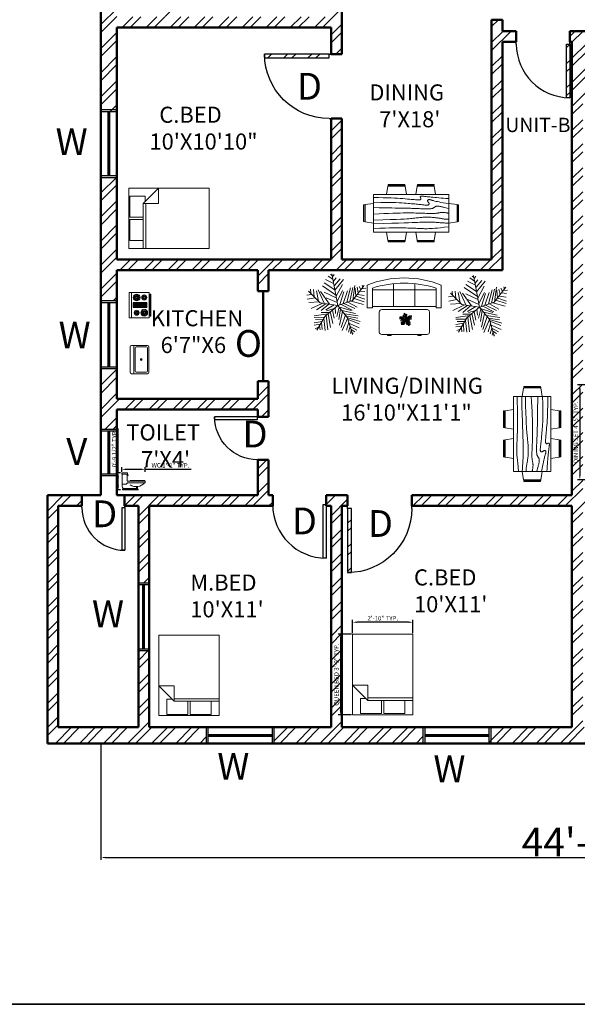
# Model space of a CAD drawing. Units: inches. Extents: x -31842 to -29388, y 18869 to 19743.
# Tile 10 of 12: x -30172 to -29859, y 18869 to 19420. Entities that reach past the tile are written whole.
import ezdxf

# ---------------------------------------------------------------- set-up
doc = ezdxf.new("R2010")
doc.units = ezdxf.units.IN
for name, color, linetype, lineweight in [('A-ANNO-DIMS', 2, 'Continuous', 18), ('A-ANNO-SYMB', 2, 'Continuous', 18), ('A-ANNO-TTLB', 7, 'Continuous', 35), ('A-AREA-IDEN', 3, 'Continuous', 18), ('A-DOOR', 3, 'Continuous', 25), ('A-FLOR-FIXT', 8, 'Continuous', 18), ('A-FURN', 8, 'Continuous', 18), ('A-GLAZ', 4, 'Continuous', 25), ('A-WALL', 7, 'Continuous', 50), ('A-WALL-PATT', 8, 'Continuous', 13), ('L-PLNT', 3, 'Continuous', 13)]:
    doc.layers.add(name, color=color, linetype=linetype, lineweight=lineweight)
doc.styles.get("Standard").update_dxf_attribs({"font": 'arial.ttf'})
doc.dimstyles.new('ISO-25', dxfattribs={"dimtxt": 2.5, "dimasz": 2.5, "dimexe": 1.25, "dimexo": 0.625, "dimtad": 1, "dimdec": 0, "dimlunit": 3, "dimtxsty": 'Standard', "dimcen": 2.5, "dimadec": 0, "dimazin": 0, "dimtfac": 1, "dimtdec": 0, "dimtmove": 0, "dimatfit": 3, "dimfxl": 1, "dimarcsym": 0})

# ---------------------------------------------------------------- blocks, each defined once
blk = doc.blocks.new('*U8')
for p, q in [((0, 0), (0, -100)), ((750, 0), (750, -100))]:
    blk.add_line(p, q)
blk.add_lwpolyline([(0, 0), (0, 750), (43.75, 750), (43.75, 0)], close=True)
blk.add_arc((0, 0), 750, 0, 90)
blk = doc.blocks.new('Bed - Queen')
for p, q in [((0, -80.00003), (0, 0)), ((0, 0), (59.99999, 0)), ((59.99999, 0), (59.99999, -80.00003)), ((7.99999, -1.2), (28.79998, -1.2)), ((7.99999, -14.4), (7.99999, -1.2)), ((28.79998, -1.2), (28.79998, -14.4)), ((31.19999, -1.2), (51.99999, -1.2)), ((31.19999, -14.4), (31.19999, -1.2)), ((51.99999, -1.2), (51.99999, -16.4)), ((0, -14.4), (44.8, -14.4)), ((44.8, -16.8), (0, -16.8)), ((59.99999, -29.6), (44.8, -14.4)), ((44.8, -14.4), (44.8, -29.6)), ((51.99999, -16.4), (46.79936, -16.4)), ((44.8, -29.6), (59.99999, -29.6)), ((59.99999, -80.00003), (0, -80.00003))]:
    blk.add_line(p, q)
blk = doc.blocks.new('Range-Oven - 30 in top')
for p, q in [((0, -3), (30, -3)), ((12, -6), (18, -6)), ((13, -20), (13, -6)), ((14, -6), (14, -20)), ((15, -20), (15, -6)), ((16, -6), (16, -20)), ((17, -20), (17, -6)), ((18, -20), (12, -20)), ((6, -24), (6, -25)), ((8, -25), (8, -24)), ((22, -25), (22, -24)), ((24, -24), (24, -25))]:
    blk.add_line(p, q)
for points in [[(0, -24), (0, 0), (30, 0), (30, -24)], [(12, -21), (12, -5), (18, -5), (18, -21)], [(2, -26), (2, -25), (28, -25), (28, -26)]]:
    blk.add_lwpolyline(points, close=True)
for centre, radius in [((6, -9), 4), ((6, -9), 3), ((6, -9), 2), ((6, -9), 1), ((24, -9), 3), ((24, -9), 2), ((24, -9), 1), ((6, -18), 3), ((6, -18), 2), ((6, -18), 1), ((24, -18), 4), ((24, -18), 3), ((24, -18), 2), ((24, -18), 1)]:
    blk.add_circle(centre, radius)
blk = doc.blocks.new('Sink-single - 30 in top')
blk.add_line((-15, -3.999996), (15, -3.999996))
for points in [[(-13.5, 0), (13.5, 0)], [(-15, -18.499996), (-15, -1.5)], [(-13.5, -17.499996), (-13.5, -6.499996)], [(-12.5, -5.499996), (12.5, -5.499996)], [(13.5, -6.499996), (13.5, -17.499996)], [(15, -1.5), (15, -18.499996)], [(13.5, -19.999996), (-13.5, -19.999996)], [(12.5, -18.499996), (-12.5, -18.499996)]]:
    blk.add_lwpolyline(points)
for radius in [1, 0.5]:
    blk.add_circle((0, -11.999996), radius)
for centre, radius, start, end in [((-13.5, -1.5), 1.5, 90, 180), ((-12.5, -6.499996), 1, 90, 180), ((12.5, -6.499996), 1, 0, 90), ((13.5, -1.5), 1.5, 0, 90), ((-13.5, -18.499996), 1.5, 180, 270), ((-12.5, -17.499996), 1, 180, 270), ((12.5, -17.499996), 1, 270, 0), ((13.5, -18.499996), 1.5, 270, 0)]:
    blk.add_arc(centre, radius, start, end)
blk = doc.blocks.new('Toilet - side')
for p, q in [((0.5, 5), (0.5, 22)), ((7.5, 22), (7.5, 12)), ((7.5, 21), (9, 21)), ((9, 20), (7.5, 20)), ((9, 21), (9, 20)), ((6, 8), (0.5, 8)), ((22, 2), (2, 2)), ((2, 2), (2, 1)), ((8, 10), (6, 8)), ((7.5, 12), (33, 12)), ((33, 10), (8, 10)), ((32.5, 13), (12, 13)), ((12, 13), (12, 12)), ((21, 4.5), (21, 2)), ((22, 2), (22, 4.5)), ((22, 1), (22, 2)), ((32.5, 12), (32.5, 13)), ((33, 12), (33, 10))]:
    blk.add_line(p, q)
for points in [[(0, 22), (0, 24), (8, 24), (8, 22)], [(1, 0), (1, 1), (23, 1), (23, 0)]]:
    blk.add_lwpolyline(points, close=True)
for centre, radius, start, end in [((3.8, 4.8), 3.26, 175.6013, 237.5288), ((20.3, 20.7), 16.2, 238.1872, 318.7702)]:
    blk.add_arc(centre, radius, start, end)
blk = doc.blocks.new('Desk - 30 x 60 in.')
for p, q in [((-26.999995, 0), (26.999995, 0)), ((-29.999995, -27), (-29.999995, -3)), ((29.999995, -3), (29.999995, -27)), ((26.999995, -30), (-26.999995, -30)), ((-20.000005, -30), (-20.000005, -31)), ((-20.000005, -31), (-16.000005, -31)), ((-16.000005, -31), (-16.000005, -30)), ((15.999995, -31), (15.999995, -30)), ((19.999995, -31), (15.999995, -31)), ((19.999995, -30), (19.999995, -31))]:
    blk.add_line(p, q)
for centre, start, end in [((-26.499995, -3.5), 98.1301, 171.8699), ((26.499995, -3.5), 8.130102, 81.8699), ((-26.499995, -26.5), 188.1301, 261.8699), ((26.499995, -26.5), 278.1301, 351.8699)]:
    blk.add_arc(centre, 3.535534, start, end)
blk = doc.blocks.new('Sofa - Roundback 7 ft.')
for p, q in [((-12.00002, -32.4421), (-12.00003, -6.5971)), ((11.99997, -32.4421), (11.99998, -6.5971)), ((-36.000027, -34), (-36.000027, -11.4696)), ((-35.999844, -13.3819), (35.9998, -13.3819)), ((35.99998, -34), (35.99998, -11.4696)), ((-36.000027, -32.4421), (35.99998, -32.4421))]:
    blk.add_line(p, q)
for points in [[(-36.000027, -34), (-42.000027, -34), (-42.000027, -8)], [(41.99998, -8), (41.99998, -34), (35.99998, -34)]]:
    blk.add_lwpolyline(points)
for centre, radius, start, end in [((0, -114.25), 114.25, 68.43141, 111.5686), ((-0.00001, -127.1968), 121.1968, 72.72033, 107.2797)]:
    blk.add_arc(centre, radius, start, end)
blk = doc.blocks.new('Dining Set - 36 x 72 in.')
for p, q in [((-22.2343, 26.00059), (-23.4847, 17.99762)), ((-22.2304, 26), (-5.7608, 26)), ((-22, 27.5), (-22.1562, 26.50042)), ((-5.8416, 26.5), (-22.1534, 26.5)), ((-22, 27.5), (-6, 27.5)), ((-5.8437, 26.49966), (-6, 27.5)), ((-4.5152, 17.99762), (-5.7655, 25.99926)), ((5.7657, 26.00059), (4.5153, 17.99762)), ((5.7696, 26), (22.2392, 26)), ((6, 27.5), (5.8438, 26.50042)), ((22.1584, 26.5), (5.8466, 26.5)), ((6, 27.5), (22, 27.5)), ((22.1563, 26.49966), (22, 27.5)), ((23.4848, 17.99762), (22.2345, 25.99926)), ((-44.0006, 8.23428), (-35.9976, 9.48474)), ((36, 18), (-36, 18)), ((-36, 18), (-36, -18)), ((44.0006, 8.23428), (35.9976, 9.48474)), ((36, -18), (36, 18)), ((-45.5, 8), (-44.5004, 8.15617)), ((-45.5, 8), (-45.5, -8)), ((-44.5, -8.15843), (-44.5, 8.15338)), ((-44, 8.23041), (-44, -8.23915)), ((44, 8.23041), (44, -8.23915)), ((44.5, -8.15843), (44.5, 8.15338)), ((45.5, 8), (44.5005, 8.15617)), ((45.5, 8), (45.5, -8)), ((-44.4997, -8.15631), (-45.5, -8)), ((-35.9976, -9.48476), (-43.9993, -8.2345)), ((35.9976, -9.48476), (43.9993, -8.2345)), ((44.4997, -8.15631), (45.5, -8)), ((-36, -18), (36, -18)), ((-22.2343, -26.0006), (-23.4847, -17.99762)), ((-4.5152, -17.99762), (-5.7655, -25.99928)), ((5.7657, -26.0006), (4.5153, -17.99762)), ((23.4848, -17.99762), (22.2345, -25.99928)), ((-22.2304, -26), (-5.7608, -26)), ((-22, -27.5), (-22.1562, -26.50044)), ((-5.8416, -26.5), (-22.1534, -26.5)), ((-22, -27.5), (-6, -27.5)), ((-5.8437, -26.49967), (-6, -27.5)), ((5.7696, -26), (22.2392, -26)), ((6, -27.5), (5.8438, -26.50044)), ((22.1584, -26.5), (5.8466, -26.5)), ((6, -27.5), (22, -27.5)), ((22.1563, -26.49967), (22, -27.5))]:
    blk.add_line(p, q)
for points in [[(-36, 15), (-31.1772, 14.97754), (-26.8079, 14.91406), (-22.8538, 14.81543), (-19.276, 14.6875), (-16.0362, 14.53613), (-13.0957, 14.36718), (-10.4159, 14.18652), (-7.9583, 14), (-5.6904, 13.81315), (-3.6035, 13.63021), (-1.6954, 13.45508), (0.0365, 13.29166), (1.5945, 13.14388), (2.9811, 13.01562), (4.1988, 12.9108), (5.25, 12.83333), (6.1393, 12.78613), (6.8802, 12.76823), (7.4883, 12.77767), (7.9792, 12.8125), (8.3685, 12.87077), (8.6719, 12.95052), (8.9049, 13.0498), (9.0833, 13.16666), (9.2205, 13.29899), (9.3216, 13.44401), (9.3895, 13.59879), (9.4271, 13.76041), (9.4373, 13.92594), (9.4232, 14.09245), (9.3875, 14.257), (9.3333, 14.41666), (9.2638, 14.56917), (9.1836, 14.71484), (9.0975, 14.85465), (9.0104, 14.98958), (8.9272, 15.1206), (8.8529, 15.2487), (8.7922, 15.37483), (8.75, 15.5), (8.7305, 15.62467), (8.7344, 15.74739), (8.7617, 15.86621), (8.8125, 15.97916), (8.8867, 16.08431), (8.9844, 16.17968), (9.1055, 16.26334), (9.25, 16.33333), (9.4189, 16.38802), (9.6172, 16.42708), (9.8506, 16.45052), (10.125, 16.45833), (10.4463, 16.45052), (10.8203, 16.42708), (11.2529, 16.38802), (11.75, 16.33333), (12.3184, 16.26318), (12.9694, 16.17838), (13.7151, 16.07991), (14.5677, 15.96875), (15.5395, 15.84586), (16.6426, 15.71224), (17.8893, 15.56884), (19.2917, 15.41666), (20.859, 15.25667), (22.5879, 15.08984), (24.4721, 14.91715), (26.5052, 14.73958), (28.6809, 14.5581), (30.9929, 14.3737), (33.4347, 14.18733), (36, 14)], [(-36, 10), (-28.9766, 10.14274), (-23.1725, 10.20442), (-18.4241, 10.19775), (-14.5677, 10.13541), (-11.4399, 10.03011), (-8.877, 9.89453), (-6.7154, 9.74137), (-4.7917, 9.58333), (-2.9698, 9.43082), (-1.2246, 9.28515), (0.4415, 9.14534), (2.026, 9.01041), (3.5266, 8.87939), (4.9408, 8.7513), (6.266, 8.62516), (7.5, 8.5), (8.6411, 8.37549), (9.6914, 8.2539), (10.6538, 8.13818), (11.5312, 8.03125), (12.3267, 7.93603), (13.043, 7.85547), (13.6831, 7.79248), (14.25, 7.75), (14.7471, 7.7303), (15.1797, 7.73307), (15.5537, 7.75732), (15.875, 7.80208), (16.1494, 7.86637), (16.3828, 7.94922), (16.5811, 8.04964), (16.75, 8.16666), (16.8944, 8.29915), (17.0143, 8.44531), (17.1089, 8.60319), (17.1771, 8.77083), (17.218, 8.94629), (17.2305, 9.1276), (17.2137, 9.31282), (17.1667, 9.5), (17.0895, 9.6875), (16.987, 9.875), (16.8649, 10.0625), (16.7292, 10.25), (16.5856, 10.4375), (16.4401, 10.625), (16.2985, 10.8125), (16.1667, 11), (16.05, 11.18733), (15.9518, 11.3737), (15.8752, 11.5581), (15.8229, 11.73958), (15.798, 11.91715), (15.8034, 12.08984), (15.842, 12.25667), (15.9167, 12.41666), (16.0295, 12.56836), (16.1784, 12.70833), (16.3605, 12.83268), (16.5729, 12.9375), (16.8127, 13.01888), (17.0768, 13.07291), (17.3625, 13.0957), (17.6667, 13.08333), (17.9894, 13.03312), (18.3418, 12.94726), (18.7382, 12.82918), (19.1927, 12.68229), (19.7195, 12.51001), (20.3327, 12.31575), (21.0465, 12.10294), (21.875, 11.875), (22.8357, 11.63354), (23.959, 11.37304), (25.2786, 11.08618), (26.8282, 10.76562), (28.6414, 10.40405), (30.752, 9.99414), (33.1936, 9.52856), (36, 9)], [(-36, 5.5), (-30.7157, 5.3348), (-26.069, 5.20963), (-21.9946, 5.11767), (-18.4271, 5.05208), (-15.3009, 5.00602), (-12.5508, 4.97265), (-10.1112, 4.94515), (-7.9167, 4.91666), (-5.909, 4.88167), (-4.0586, 4.83984), (-2.3429, 4.79215), (-0.7396, 4.73958), (0.7739, 4.6831), (2.22, 4.6237), (3.6213, 4.56233), (5, 4.5), (6.373, 4.43782), (7.7344, 4.3776), (9.0723, 4.32129), (10.375, 4.27083), (11.6309, 4.22819), (12.8281, 4.19531), (13.9551, 4.17415), (15, 4.16666), (15.954, 4.17448), (16.819, 4.19791), (17.6001, 4.23698), (18.3021, 4.29166), (18.9299, 4.36198), (19.4883, 4.44791), (19.9823, 4.54948), (20.4167, 4.66666), (20.7969, 4.79899), (21.1302, 4.94401), (21.4245, 5.09879), (21.6875, 5.26041), (21.9271, 5.42594), (22.1511, 5.59245), (22.3672, 5.757), (22.5834, 5.91666), (22.8065, 6.06868), (23.0404, 6.21093), (23.2879, 6.34147), (23.5521, 6.45833), (23.8358, 6.55957), (24.142, 6.64323), (24.4735, 6.70735), (24.8334, 6.75), (25.2235, 6.76969), (25.642, 6.76692), (26.0858, 6.74267), (26.5521, 6.69791), (27.0379, 6.63362), (27.5404, 6.55078), (28.0565, 6.45036), (28.5834, 6.33333), (29.1242, 6.19987), (29.7071, 6.04687), (30.3661, 5.87044), (31.1354, 5.66666), (32.0493, 5.43164), (33.142, 5.16146), (34.4475, 4.85221), (36, 4.5)], [(-36, -1), (-30.7915, -0.6591), (-26.0195, -0.38216), (-21.6519, -0.16284), (-17.6563, 0.00521), (-14.0005, 0.12833), (-10.6523, 0.21289), (-7.5796, 0.26522), (-4.75, 0.29166), (-2.134, 0.29793), (0.2878, 0.28711), (2.5317, 0.26163), (4.6146, 0.22396), (6.5529, 0.17651), (8.3633, 0.12174), (10.0623, 0.06209), (11.6667, 0), (13.1899, -0.06201), (14.6341, -0.1211), (15.9982, -0.17432), (17.2813, -0.21875), (18.4823, -0.25147), (19.6003, -0.26953), (20.6343, -0.27002), (21.5834, -0.25), (22.4481, -0.20768), (23.2357, -0.14584), (23.9549, -0.06836), (24.6146, 0.02083), (25.2235, 0.11784), (25.7904, 0.21875), (26.3241, 0.31966), (26.8334, 0.41666), (27.3265, 0.50618), (27.8099, 0.58593), (28.2894, 0.65397), (28.7709, 0.70833), (29.2601, 0.74707), (29.763, 0.76823), (30.2855, 0.76985), (30.8334, 0.75), (31.4088, 0.70784), (31.9994, 0.64713), (32.589, 0.57275), (33.1615, 0.48958), (33.7008, 0.4025), (34.1908, 0.3164), (34.6153, 0.23616), (34.9584, 0.16666), (35.2099, 0.11165), (35.3848, 0.07031), (35.504, 0.04069), (35.5886, 0.02083), (35.6594, 0.00879), (35.7377, 0.0026), (35.8442, 0.00032), (36, 0)], [(-36, -6.5), (-27.1843, -6.31267), (-20.084, -6.1263), (-14.469, -5.9419), (-10.1094, -5.76042), (-6.7752, -5.58285), (-4.2363, -5.41016), (-2.2629, -5.24333), (-0.625, -5.08334), (0.8708, -4.93099), (2.2715, -4.78646), (3.5872, -4.64974), (4.8281, -4.52084), (6.0046, -4.39974), (7.127, -4.28646), (8.2053, -4.18099), (9.25, -4.08334), (10.2705, -3.99382), (11.2734, -3.91407), (12.2647, -3.84603), (13.25, -3.79167), (14.2354, -3.75293), (15.2266, -3.73177), (16.2295, -3.73015), (17.25, -3.75), (18.2912, -3.79248), (19.3451, -3.85547), (20.4009, -3.93604), (21.4479, -4.03125), (22.4754, -4.13819), (23.4727, -4.25391), (24.4289, -4.37549), (25.3334, -4.5), (26.1785, -4.62492), (26.9694, -4.74935), (27.7145, -4.87281), (28.4219, -4.99479), (29.1, -5.11483), (29.7572, -5.23242), (30.4016, -5.34709), (31.0417, -5.45834), (31.6837, -5.56437), (32.3262, -5.65821), (32.9658, -5.73153), (33.599, -5.77604), (34.2224, -5.78345), (34.8327, -5.74545), (35.4264, -5.65373), (36, -5.5)], [(-36, -10), (-26.4022, -9.81299), (-18.4675, -9.62891), (-11.9839, -9.45069), (-6.7396, -9.28125), (-2.5226, -9.12354), (0.8789, -8.98047), (3.6769, -8.85498), (6.0833, -8.75), (8.2767, -8.66765), (10.3021, -8.60677), (12.1712, -8.56543), (13.8958, -8.54167), (15.4876, -8.53353), (16.9583, -8.53907), (18.3197, -8.55632), (19.5834, -8.58334), (20.7616, -8.61841), (21.8685, -8.66081), (22.9188, -8.71004), (23.9271, -8.76563), (24.9081, -8.82707), (25.8763, -8.89388), (26.8465, -8.96558), (27.8334, -9.04167), (28.8474, -9.12118), (29.8828, -9.20117), (30.93, -9.27824), (31.9792, -9.34896), (33.0205, -9.40991), (34.0443, -9.45768), (35.0407, -9.48885), (36, -9.5)], [(-36, -14.5), (-30.0881, -14.33513), (-25.0332, -14.21224), (-20.7312, -14.12647), (-17.0781, -14.07292), (-13.97, -14.04671), (-11.3027, -14.04297), (-8.9724, -14.05681), (-6.875, -14.08334), (-4.9224, -14.11833), (-3.0905, -14.16016), (-1.3709, -14.20785), (0.2448, -14.26042), (1.7647, -14.3169), (3.1973, -14.3763), (4.5507, -14.43767), (5.8333, -14.5), (7.0554, -14.5621), (8.235, -14.62175), (9.3922, -14.67652), (10.5469, -14.72396), (11.7192, -14.76164), (12.929, -14.78711), (14.1965, -14.79794), (15.5417, -14.79167), (16.9933, -14.76424), (18.6152, -14.70508), (20.4804, -14.60197), (22.6615, -14.44271), (25.2312, -14.21509), (28.2624, -13.9069), (31.8277, -13.50594), (36, -13)]]:
    blk.add_lwpolyline(points)
blk = doc.blocks.new('*U122')
for p, q in [((-258.7244, 1362.456), (-332.3336, 1421.4348)), ((0, 0), (-266.7, 1447.8)), ((-231.1146, 1315.2628), (-166.7002, 1421.4348)), ((-129.8956, 713.6638), (-626.7704, 1032.1544)), ((-185.1152, 1008.5578), (-553.1612, 1185.4942)), ((-221.9198, 1197.3052), (-433.5526, 1338.8594)), ((-194.31, 1102.9442), (-65.4812, 1256.284)), ((-148.3106, 914.1968), (118.5418, 1220.9018)), ((-129.8956, 701.8528), (265.7602, 1185.4942)), ((-74.7014, 418.7444), (219.7608, 961.39)), ((685.8, 228.6), (1219.2, 914.4)), ((689.0258, 230.0224), (790.2448, 914.1968)), ((1121.4862, 925.9824), (1149.0706, 831.6214)), ((-1206.4492, 501.3198), (-1418.082, 465.9376)), ((-800.1, 114.3), (-1333.5, 647.7)), ((-1234.059, 536.7274), (-1252.4486, 737.2604)), ((-1105.2302, 725.4494), (-1077.6458, 395.1732)), ((-976.4268, 666.4706), (-884.4026, 194.6402)), ((-902.8176, 713.6638), (-617.5756, 100.2538)), ((-369.1382, 53.086), (-783.1836, 642.874)), ((-93.091, 489.5342), (-700.3796, 902.3858)), ((-617.5756, 607.4918), (-74.7014, 347.98)), ((-28.6766, 171.0436), (228.9556, 678.2816)), ((100.1268, 41.275), (284.1498, 619.2774)), ((256.5654, 88.4682), (449.7832, 666.4706)), ((412.9786, 147.447), (587.8068, 796.2392)), ((560.197, 182.8292), (698.2206, 819.8358)), ((808.6344, 784.4282), (827.0494, 418.7444)), ((891.4384, 831.6214), (946.658, 572.1096)), ((919.0482, 501.3198), (1222.6798, 454.152)), ((983.4626, 867.0036), (1066.2666, 725.4494)), ((1029.462, 654.685), (1241.0948, 631.0884)), ((1112.2914, 760.8316), (1296.3144, 784.4282)), ((-1031.621, 347.98), (-1399.667, 277.1902)), ((-847.598, 159.2326), (-1326.0578, 135.636)), ((-718.7946, 88.4682), (-1215.644, -147.447)), ((-543.9664, 76.6572), (-967.2066, -206.4512)), ((0, 0), (-800.1, 114.3)), ((-405.9428, 53.086), (-764.794, -241.8334)), ((0, 0), (-571.5, -495.3)), ((-166.7002, 29.4894), (-543.9664, -206.4512)), ((-525.5514, 347.98), (-28.6766, 123.8504)), ((0, 0), (685.8, 228.6)), ((0, 0), (457.2, -571.5)), ((164.5412, 41.275), (661.416, -218.2368)), ((284.1498, 88.4682), (781.0246, -147.447)), ((458.978, 147.447), (891.4384, -88.4682)), ((615.4166, 194.6402), (1185.8752, 41.275)), ((753.4148, 312.5978), (1222.6798, 159.2326)), ((845.439, 418.7444), (1241.0948, 277.1902)), ((-442.7474, -383.3876), (-1086.8406, -477.7486)), ((-387.5278, -324.4088), (-764.794, -324.4088)), ((-166.7002, -147.447), (-507.1618, -253.619)), ((-433.5526, -383.3876), (-323.1134, -1020.3688)), ((-341.5284, -289.0012), (-221.9198, -831.6214)), ((-240.3094, -218.2368), (-157.5054, -595.7062)), ((-120.7008, -88.4682), (-93.091, -371.5766)), ((63.3222, -76.6826), (-37.8714, -513.1308)), ((44.9326, -64.897), (615.4166, -241.8334)), ((127.7366, -159.258), (54.1274, -654.685)), ((228.9556, -289.0012), (90.932, -914.1968)), ((357.759, -430.5554), (164.5412, -1020.3688)), ((192.151, -230.0224), (817.8292, -371.5766)), ((311.7596, -383.3876), (937.4378, -477.7486)), ((-718.7946, -737.2604), (-1086.8406, -796.2392)), ((-617.5756, -548.5384), (-1077.6458, -560.324)), ((-783.1836, -867.029), (-1077.6458, -902.4112)), ((-681.9646, -666.496), (-1022.4262, -654.685)), ((-571.5, -495.3), (-952.5, -1143)), ((-737.1842, -784.4536), (-709.5744, -1114.7298)), ((-635.9652, -607.5172), (-580.771, -1150.1374)), ((-525.5514, -465.963), (-451.9422, -1126.5408)), ((458.978, -572.1096), (210.5406, -1161.923)), ((514.1976, -772.6426), (403.7838, -1138.3264)), ((412.9786, -501.3452), (919.0482, -583.9206)), ((457.2, -571.5), (685.8, -1333.5)), ((468.1982, -572.1096), (1029.462, -737.2604)), ((486.5878, -642.8994), (983.4626, -843.4324)), ((541.8074, -831.6214), (992.6574, -1032.1544)), ((-875.2078, -1008.5832), (-1040.8412, -1079.3476)), ((-829.2084, -937.7934), (-810.7934, -1126.5408)), ((578.612, -961.39), (495.7826, -1232.7128)), ((578.612, -973.1756), (873.0488, -1138.3264)), ((624.6114, -1161.923), (587.8068, -1291.6916)), ((624.6114, -1102.9442), (781.0246, -1209.1162)), ((679.8056, -1268.095), (716.6102, -1291.6916))]:
    blk.add_line(p, q)
blk = doc.blocks.new('*D212')
at = {"layer": 'A-ANNO-DIMS', "color": 0, "lineweight": -2, "transparency": 16777216}
for p, q in [((-30126.5, 19014.34), (-30126.5, 18949.8)), ((-29594.5, 19014.34), (-29594.5, 18949.8)), ((-30124, 18951.05), (-29597, 18951.05))]:
    blk.add_line(p, q, dxfattribs=at)
at = {"layer": 'A-ANNO-DIMS', "color": 0, "transparency": 16777216}
for points in [[(-30124, 18951.47), (-30124, 18950.64), (-30126.5, 18951.05)], [(-29597, 18951.47), (-29597, 18950.64), (-29594.5, 18951.05)]]:
    blk.add_solid(points, dxfattribs=at)
at = {"layer": 'Defpoints', "color": 0, "transparency": 16777216}
for p in [(-30126.5, 19014.96), (-29594.5, 19014.96), (-29594.5, 18951.05)]:
    blk.add_point(p, dxfattribs=at)
at = {"layer": 'A-ANNO-DIMS', "color": 0, "transparency": 16777216, "insert": (-29860.5, 18959.68), "char_height": 2.5, "attachment_point": 5}
blk.add_mtext('{\\H6.4x;44\'-4"}', dxfattribs=at)
blk = doc.blocks.new('WIN-3FT')
for p, q in [((0, 36), (9, 36)), ((4, 0), (4, 36)), ((4.5, 0), (4.5, 36)), ((5, 0), (5, 36)), ((0, 0), (9, 0))]:
    blk.add_line(p, q)
blk = doc.blocks.new('WIN-3FT-B')
for p, q in [((0, 36), (6, 36)), ((2.5, 0), (2.5, 36)), ((3, 0), (3, 36)), ((3.5, 0), (3.5, 36)), ((0, 0), (6, 0))]:
    blk.add_line(p, q)
blk = doc.blocks.new('WIN-2FT')
for p, q in [((0, 24), (9, 24)), ((4, 0), (4, 24)), ((4.5, 0), (4.5, 24)), ((5, 0), (5, 24)), ((0, 0), (9, 0))]:
    blk.add_line(p, q)
blk = doc.blocks.new('*D223')
at = {"layer": 'A-ANNO-DIMS', "color": 0, "lineweight": -2, "transparency": 16777216}
for p, q in [((-29986.05, 19076.06), (-29993.45, 19076.06)), ((-29992.2, 19073.56), (-29992.2, 19033.45)), ((-29986.05, 19030.95), (-29993.45, 19030.95))]:
    blk.add_line(p, q, dxfattribs=at)
at = {"layer": 'A-ANNO-DIMS', "color": 0, "transparency": 16777216}
for points in [[(-29992.61, 19073.56), (-29991.78, 19073.56), (-29992.2, 19076.06)], [(-29992.61, 19033.45), (-29991.78, 19033.45), (-29992.2, 19030.95)]]:
    blk.add_solid(points, dxfattribs=at)
at = {"layer": 'Defpoints', "color": 0, "transparency": 16777216}
for p in [(-29985.43, 19076.06), (-29992.2, 19030.95), (-29985.43, 19030.95)]:
    blk.add_point(p, dxfattribs=at)
at = {"layer": 'A-ANNO-DIMS', "color": 0, "transparency": 16777216, "insert": (-29994.19, 19053.51), "char_height": 2.5, "attachment_point": 5, "rotation": 90}
blk.add_mtext('QUEEN BED 3\'-9" TYP.', dxfattribs=at)
blk = doc.blocks.new('*D224')
at = {"layer": 'A-ANNO-DIMS', "color": 0, "lineweight": -2, "transparency": 16777216}
for p, q in [((-29985.43, 19076.68), (-29985.43, 19084.08)), ((-29954.1, 19082.83), (-29982.93, 19082.83)), ((-29951.6, 19076.68), (-29951.6, 19084.08))]:
    blk.add_line(p, q, dxfattribs=at)
at = {"layer": 'A-ANNO-DIMS', "color": 0, "transparency": 16777216}
for points in [[(-29982.93, 19083.24), (-29982.93, 19082.41), (-29985.43, 19082.83)], [(-29954.1, 19083.24), (-29954.1, 19082.41), (-29951.6, 19082.83)]]:
    blk.add_solid(points, dxfattribs=at)
at = {"layer": 'Defpoints', "color": 0, "transparency": 16777216}
for p in [(-29985.43, 19082.83), (-29985.43, 19076.06), (-29951.6, 19076.06)]:
    blk.add_point(p, dxfattribs=at)
at = {"layer": 'A-ANNO-DIMS', "color": 0, "transparency": 16777216, "insert": (-29968.51, 19084.73), "char_height": 2.5, "attachment_point": 5}
blk.add_mtext('2\'-10" TYP.', dxfattribs=at)
blk = doc.blocks.new('*D229')
at = {"layer": 'A-ANNO-DIMS', "color": 0, "lineweight": -2, "transparency": 16777216}
for p, q in [((-30114.79, 19167.13), (-30114.79, 19169.72)), ((-30112.29, 19168.47), (-30104.21, 19168.47)), ((-30101.71, 19167.13), (-30101.71, 19169.72)), ((-30101.71, 19168.47), (-30075.83, 19168.47))]:
    blk.add_line(p, q, dxfattribs=at)
at = {"layer": 'A-ANNO-DIMS', "color": 0, "transparency": 16777216}
for points in [[(-30112.29, 19168.89), (-30112.29, 19168.05), (-30114.79, 19168.47)], [(-30104.21, 19168.89), (-30104.21, 19168.05), (-30101.71, 19168.47)]]:
    blk.add_solid(points, dxfattribs=at)
at = {"layer": 'Defpoints', "color": 0, "transparency": 16777216}
for p in [(-30114.79, 19166.51), (-30101.71, 19168.47), (-30101.71, 19166.51)]:
    blk.add_point(p, dxfattribs=at)
at = {"layer": 'A-ANNO-DIMS', "color": 0, "transparency": 16777216, "insert": (-30087.52, 19170.39), "char_height": 2.5, "attachment_point": 5}
blk.add_mtext('WC 1\'-1" TYP.', dxfattribs=at)
blk = doc.blocks.new('*D230')
at = {"layer": 'A-ANNO-DIMS', "color": 0, "lineweight": -2, "transparency": 16777216}
for p, q in [((-30116.76, 19166.51), (-30116.76, 19191.32)), ((-30115.42, 19166.51), (-30118.01, 19166.51)), ((-30116.76, 19159.49), (-30116.76, 19164.01)), ((-30115.42, 19156.99), (-30118.01, 19156.99))]:
    blk.add_line(p, q, dxfattribs=at)
at = {"layer": 'A-ANNO-DIMS', "color": 0, "transparency": 16777216}
for points in [[(-30117.17, 19164.01), (-30116.34, 19164.01), (-30116.76, 19166.51)], [(-30117.17, 19159.49), (-30116.34, 19159.49), (-30116.76, 19156.99)]]:
    blk.add_solid(points, dxfattribs=at)
at = {"layer": 'Defpoints', "color": 0, "transparency": 16777216}
for p in [(-30116.76, 19166.51), (-30114.79, 19166.51), (-30114.79, 19156.99)]:
    blk.add_point(p, dxfattribs=at)
at = {"layer": 'A-ANNO-DIMS', "color": 0, "transparency": 16777216, "insert": (-30118.67, 19180.16), "char_height": 2.5, "attachment_point": 5, "rotation": 90}
blk.add_mtext('0\'-9 1/2" TYP.', dxfattribs=at)
blk = doc.blocks.new('*D245')
at = {"layer": 'A-ANNO-DIMS', "color": 0, "lineweight": -2, "transparency": 16777216}
for p, q in [((-29850.74, 19215.8), (-29859.34, 19215.8)), ((-29858.09, 19213.3), (-29858.09, 19165.11)), ((-29850.74, 19162.61), (-29859.34, 19162.61))]:
    blk.add_line(p, q, dxfattribs=at)
at = {"layer": 'A-ANNO-DIMS', "color": 0, "transparency": 16777216}
for points in [[(-29858.51, 19213.3), (-29857.67, 19213.3), (-29858.09, 19215.8)], [(-29858.51, 19165.11), (-29857.67, 19165.11), (-29858.09, 19162.61)]]:
    blk.add_solid(points, dxfattribs=at)
at = {"layer": 'Defpoints', "color": 0, "transparency": 16777216}
for p in [(-29850.11, 19215.8), (-29858.09, 19162.61), (-29850.11, 19162.61)]:
    blk.add_point(p, dxfattribs=at)
at = {"layer": 'A-ANNO-DIMS', "color": 0, "transparency": 16777216, "insert": (-29860.01, 19189.21), "char_height": 2.5, "attachment_point": 5, "rotation": 90}
blk.add_mtext('DINING SET 4\'-5" TYP.', dxfattribs=at)

msp = doc.modelspace()

# ---------------------------------------------------------------- hatches: boundary and pattern name
at = {"layer": 'A-WALL-PATT'}
h = msp.add_hatch(dxfattribs=at)
h.set_pattern_fill('ANSI32', color=256)
h.paths.add_polyline_path([(-29790.5, 19614.96), (-29841.5, 19614.96), (-29841.5, 19605.96), (-29819.5, 19605.96), (-29819.5, 19455.01), (-29813.5, 19455.01), (-29813.5, 19491.96), (-29800.11, 19491.96), (-29800.11, 19497.96), (-29813.5, 19497.96), (-29813.5, 19605.96), (-29790.5, 19605.96)])
h.paths.add_polyline_path([(-29879.5, 19614.96), (-29930.5, 19614.96), (-29930.5, 19605.96), (-29907.5, 19605.96), (-29907.5, 19497.96), (-29922.61, 19497.96), (-29922.61, 19491.96), (-29907.5, 19491.96), (-29907.5, 19456.33), (-29903.21, 19456.33), (-29901.5, 19456.31), (-29901.5, 19605.96), (-29879.5, 19605.96)])
h.paths.add_polyline_path([(-29968.5, 19614.96), (-29991.5, 19614.96), (-29991.5, 19656.96), (-30126.5, 19656.96), (-30126.5, 19559.96), (-30117.5, 19559.96), (-30117.5, 19605.96), (-30029.48, 19605.96), (-30029.48, 19614.96), (-30117.5, 19614.96), (-30117.5, 19650.96), (-29997.5, 19650.96), (-29997.5, 19614.96), (-30005.48, 19614.96), (-30005.48, 19605.96), (-29997.5, 19605.96), (-29997.5, 19549.04), (-29991.5, 19549.04), (-29991.5, 19605.96), (-29968.5, 19605.96)])
h.paths.add_polyline_path([(-29716.42, 19614.96), (-29723.5, 19614.96), (-29723.5, 19650.96), (-29603.5, 19650.96), (-29603.5, 19614.96), (-29692.42, 19614.96), (-29692.42, 19605.96), (-29687.14, 19605.96), (-29603.5, 19605.96), (-29603.5, 19559.96), (-29594.5, 19559.96), (-29594.5, 19656.96), (-29729.5, 19656.96), (-29729.5, 19614.96), (-29752.5, 19614.96), (-29752.5, 19605.96), (-29729.5, 19605.96), (-29729.5, 19551.13), (-29723.5, 19551.13), (-29723.5, 19605.96), (-29716.42, 19605.96)])
h.paths.add_polyline_path([(-29628.39, 19472.82), (-29628.34, 19475.96), (-29723.5, 19475.96), (-29723.5, 19515.13), (-29729.5, 19515.13), (-29729.5, 19497.96), (-29744.93, 19497.96), (-29744.93, 19491.96), (-29729.5, 19491.96), (-29729.5, 19460.98), (-29723.5, 19460.98), (-29723.5, 19469.96), (-29636.5, 19469.96), (-29636.5, 19458.96), (-29630.5, 19458.96), (-29630.5, 19469.96), (-29628.39, 19469.96)])
h.paths.add_polyline_path([(-29594.5, 19521.96), (-29603.5, 19521.96), (-29603.5, 19475.96), (-29604.34, 19475.96), (-29604.34, 19469.96), (-29603.5, 19469.96), (-29603.5, 19421.96), (-29630.5, 19421.96), (-29630.5, 19432.96), (-29636.5, 19432.96), (-29636.5, 19421.96), (-29723.5, 19421.96), (-29723.5, 19436.98), (-29729.5, 19436.98), (-29729.5, 19396.75), (-29723.5, 19396.75), (-29723.5, 19415.96), (-29603.5, 19415.96), (-29603.5, 19369.96), (-29594.5, 19369.96)])
h.paths.add_polyline_path([(-29594.5, 19331.96), (-29603.5, 19331.96), (-29603.5, 19285.96), (-29723.5, 19285.96), (-29723.5, 19360.75), (-29729.5, 19360.75), (-29729.5, 19285.96), (-29813.5, 19285.96), (-29813.5, 19419.01), (-29819.5, 19419.01), (-29819.5, 19413.96), (-29825.38, 19413.96), (-29825.38, 19407.96), (-29819.5, 19407.96), (-29819.5, 19279.96), (-29688.5, 19279.96), (-29688.5, 19267.87), (-29682.5, 19267.87), (-29682.5, 19279.96), (-29603.5, 19279.96), (-29603.5, 19262.96), (-29594.5, 19262.96)])
h.paths.add_polyline_path([(-29594.5, 19224.96), (-29603.5, 19224.96), (-29603.5, 19207.96), (-29682.5, 19207.96), (-29682.5, 19219.98), (-29688.5, 19219.98), (-29688.5, 19194.76), (-29682.5, 19194.76), (-29682.5, 19201.96), (-29603.5, 19201.96), (-29603.5, 19190.96), (-29594.5, 19190.96)])
h.paths.add_polyline_path([(-29564.5, 19153.96), (-29584.31, 19153.96), (-29584.31, 19147.96), (-29570.5, 19147.96), (-29570.5, 19023.96), (-29615.5, 19023.96), (-29615.5, 19066.96), (-29621.5, 19066.96), (-29621.5, 19023.96), (-29653.5, 19023.96), (-29653.5, 19014.96), (-29564.5, 19014.96)])
h.paths.add_polyline_path([(-29608.31, 19153.96), (-29682.5, 19153.96), (-29682.5, 19170.76), (-29688.5, 19170.76), (-29688.5, 19153.96), (-29691.71, 19153.96), (-29691.71, 19147.96), (-29621.5, 19147.96), (-29621.5, 19104.96), (-29615.5, 19104.96), (-29615.5, 19147.96), (-29608.31, 19147.96)])
h.paths.add_polyline_path([(-29721.71, 19153.96), (-29739.81, 19153.96), (-29739.81, 19147.96), (-29729.5, 19147.96), (-29729.5, 19023.96), (-29774, 19023.96), (-29774, 19014.96), (-29691.5, 19014.96), (-29691.5, 19023.96), (-29723.5, 19023.96), (-29723.5, 19147.96), (-29721.71, 19147.96)])
h.paths.add_polyline_path([(-29946, 19023.96), (-29991.5, 19023.96), (-29991.5, 19147.96), (-29988.28, 19147.96), (-29988.28, 19153.96), (-30000.21, 19153.96), (-30000.21, 19147.96), (-29997.5, 19147.96), (-29997.5, 19023.96), (-30029.5, 19023.96), (-30029.5, 19014.96), (-29946, 19014.96)])
h.paths.add_polyline_path([(-30067.5, 19023.96), (-30099.5, 19023.96), (-30099.5, 19066.96), (-30105.5, 19066.96), (-30105.5, 19023.96), (-30150.5, 19023.96), (-30150.5, 19147.96), (-30137.18, 19147.96), (-30137.18, 19153.96), (-30156.5, 19153.96), (-30156.5, 19014.96), (-30067.5, 19014.96)])
h.paths.add_polyline_path([(-30099.5, 19147.96), (-30030.21, 19147.96), (-30030.21, 19153.96), (-30032.5, 19153.96), (-30032.5, 19173.83), (-30038.5, 19173.83), (-30038.5, 19153.96), (-30113.18, 19153.96), (-30113.18, 19147.96), (-30105.5, 19147.96), (-30105.5, 19104.96), (-30099.5, 19104.96)])
h.paths.add_polyline_path([(-30032.5, 19217.89), (-30038.5, 19217.89), (-30038.5, 19207.96), (-30117.5, 19207.96), (-30117.5, 19224.96), (-30126.5, 19224.96), (-30126.5, 19190.96), (-30117.5, 19190.96), (-30117.5, 19201.96), (-30038.5, 19201.96), (-30038.5, 19197.83), (-30032.5, 19197.83)])
h.paths.add_polyline_path([(-29901.5, 19407.96), (-29893.72, 19407.96), (-29893.72, 19413.96), (-29901.5, 19413.96), (-29901.5, 19420.31), (-29907.5, 19420.31), (-29907.5, 19285.96), (-29991.5, 19285.96), (-29991.5, 19365.01), (-29997.5, 19365.01), (-29997.5, 19285.96), (-30117.5, 19285.96), (-30117.5, 19331.96), (-30126.5, 19331.96), (-30126.5, 19262.96), (-30117.5, 19262.96), (-30117.5, 19279.96), (-30038.5, 19279.96), (-30038.5, 19268.29), (-30032.5, 19268.29), (-30032.5, 19279.96), (-29901.5, 19279.96)])
h.paths.add_polyline_path([(-29863.72, 19413.96), (-29855.38, 19413.96), (-29855.38, 19406.96), (-29853.63, 19406.96), (-29853.63, 19376.96), (-29856.5, 19376.96), (-29856.5, 19153.96), (-29775.81, 19153.96), (-29775.81, 19148.44, 0.39722), (-29741.97, 19112.57), (-29741.97, 19148.44), (-29739.88, 19148.44), (-29739.88, 19112.51), (-29741.97, 19112.51), (-29741.97, 19112.57, -0.393359), (-29775.8, 19147.96), (-29856.5, 19147.96), (-29856.5, 19023.96), (-29811, 19023.96), (-29811, 19014.96), (-29909, 19014.96), (-29909, 19018.96), (-29945, 19018.96), (-29945, 19019.96), (-29909, 19019.96), (-29909, 19023.96), (-29862.5, 19023.96), (-29862.5, 19147.96), (-29901.5, 19147.96), (-29952.22, 19147.96), (-29952.22, 19146.6, -0.39722), (-29986.12, 19110.67), (-29986.12, 19110.6), (-29988.22, 19110.6), (-29988.22, 19146.6), (-29986.12, 19146.6), (-29986.12, 19110.67, 0.39722), (-29952.22, 19146.6), (-29952.22, 19147.96), (-29952.28, 19147.96), (-29952.28, 19153.96), (-29901.5, 19153.96), (-29862.5, 19153.96), (-29862.5, 19407.96), (-29863.72, 19407.96), (-29863.72, 19406.62), (-29863.72, 19376.63), (-29865.47, 19376.63), (-29865.47, 19406.62), (-29863.72, 19406.62), (-29863.72, 19407.96), (-29863.72, 19407.96)])
h.paths.add_polyline_path([(-30021.02, 19461.17), (-30021.06, 19461.17), (-30021.06, 19462.57), (-29997.02, 19462.57), (-29997.02, 19461.17), (-30021.02, 19461.17, 0.386026), (-29997.95, 19438.55), (-29991.5, 19438.55), (-29991.5, 19401.01), (-29998.66, 19401.01), (-29998.66, 19398.9), (-30034.72, 19398.9), (-30034.72, 19401.01), (-29997.5, 19401.01), (-29997.5, 19415.96), (-30117.5, 19415.96), (-30117.5, 19368.96), (-30121.5, 19368.96), (-30121.5, 19332.96), (-30122.5, 19332.96), (-30122.5, 19368.96), (-30126.5, 19368.96), (-30126.5, 19522.96), (-30117.5, 19522.96), (-30117.5, 19475.96), (-30116.52, 19475.96), (-30116.52, 19469.92, 0.39722), (-30093.92, 19445.96), (-30093.92, 19469.92), (-30092.52, 19469.92), (-30092.52, 19445.92), (-30093.92, 19445.92), (-30093.92, 19445.96, -0.39722), (-30116.52, 19469.92), (-30117.5, 19421.96), (-30090.5, 19421.96), (-30090.5, 19433.96), (-30084.5, 19433.96), (-30084.5, 19421.96), (-29997.5, 19421.96), (-29997.5, 19438.54, -0.391477)])
h.paths.add_polyline_path([(-29991.5, 19491.96), (-29980.66, 19491.96), (-29980.66, 19497.96), (-29991.5, 19497.96), (-29991.5, 19513.04), (-29997.5, 19513.04), (-29997.5, 19475.96), (-30092.52, 19475.96), (-30092.52, 19469.96), (-30090.5, 19469.96), (-30090.5, 19458.96), (-30084.5, 19458.96), (-30084.5, 19469.96), (-29997.5, 19469.96), (-29997.5, 19462.57), (-29997.02, 19462.57), (-29991.5, 19462.55)])
h.paths.add_polyline_path([(-29857.76, 19352.86), (-29815.8, 19352.86), (-29815.8, 19369.38), (-29857.76, 19369.38)], flags=24)

# ---------------------------------------------------------------- linework, layer by layer
at = {"layer": 'A-ANNO-TTLB'}
msp.add_lwpolyline([(-31842.18, 19743.36), (-29387.67, 19743.36), (-29387.67, 18868.82), (-31842.18, 18868.82)], close=True, dxfattribs=at)
at = {"layer": 'A-GLAZ'}
for p, q in [((-30126.5, 19369.96), (-30117.5, 19369.96)), ((-30126.5, 19331.96), (-30117.5, 19331.96)), ((-30126.5, 19262.96), (-30117.5, 19262.96)), ((-30126.5, 19224.96), (-30117.5, 19224.96)), ((-30126.5, 19190.96), (-30117.5, 19190.96)), ((-30126.5, 19164.96), (-30117.5, 19164.96)), ((-30105.5, 19104.96), (-30099.5, 19104.96)), ((-30105.5, 19066.96), (-30099.5, 19066.96)), ((-30067.5, 19023.96), (-30067.5, 19014.96)), ((-30029.5, 19023.96), (-30029.5, 19014.96)), ((-29946, 19023.96), (-29946, 19014.96)), ((-29908, 19023.96), (-29908, 19014.96))]:
    msp.add_line(p, q, dxfattribs=at)
at = {"layer": 'A-WALL'}
for p, q in [((-30126.5, 19153.96), (-30126.5, 19656.96)), ((-29991.5, 19401.01), (-29991.5, 19438.55)), ((-29907.5, 19285.96), (-29907.5, 19420.31)), ((-29907.5, 19420.31), (-29901.5, 19420.31)), ((-29901.5, 19413.96), (-29901.5, 19420.31)), ((-30117.5, 19415.96), (-29997.5, 19415.96)), ((-30117.5, 19285.96), (-30117.5, 19415.96)), ((-29997.5, 19401.01), (-29997.5, 19415.96)), ((-29901.5, 19413.96), (-29893.72, 19413.96)), ((-29893.72, 19407.96), (-29893.72, 19413.96)), ((-29863.72, 19407.96), (-29863.72, 19413.96)), ((-29863.72, 19413.96), (-29855.38, 19413.96)), ((-29901.5, 19279.96), (-29901.5, 19407.96)), ((-29901.5, 19407.96), (-29893.72, 19407.96)), ((-29863.72, 19407.96), (-29862.5, 19407.96)), ((-29862.5, 19153.96), (-29862.5, 19407.96)), ((-29997.5, 19401.01), (-29991.5, 19401.01)), ((-29997.5, 19285.96), (-29997.5, 19365.01)), ((-29997.5, 19365.01), (-29991.5, 19365.01)), ((-29991.5, 19285.96), (-29991.5, 19365.01)), ((-30117.5, 19285.96), (-29997.5, 19285.96)), ((-29991.5, 19285.96), (-29907.5, 19285.96)), ((-30117.5, 19279.96), (-30038.5, 19279.96)), ((-30117.5, 19207.96), (-30117.5, 19279.96)), ((-30038.5, 19268.29), (-30038.5, 19279.96)), ((-30032.5, 19279.96), (-29901.5, 19279.96)), ((-30032.5, 19268.29), (-30032.5, 19279.96)), ((-30038.5, 19268.29), (-30032.5, 19268.29)), ((-30035.5, 19268.29), (-30035.5, 19217.89)), ((-30038.5, 19207.96), (-30038.5, 19217.89)), ((-30038.5, 19217.89), (-30032.5, 19217.89)), ((-30032.5, 19197.83), (-30032.5, 19217.89)), ((-30117.5, 19207.96), (-30038.5, 19207.96)), ((-30117.5, 19153.96), (-30117.5, 19201.96)), ((-30117.5, 19201.96), (-30038.5, 19201.96)), ((-30038.5, 19197.83), (-30038.5, 19201.96)), ((-30038.5, 19197.83), (-30032.5, 19197.83)), ((-30038.5, 19153.96), (-30038.5, 19173.83)), ((-30038.5, 19173.83), (-30032.5, 19173.83)), ((-30032.5, 19153.96), (-30032.5, 19173.83)), ((-30156.5, 19153.96), (-30126.5, 19153.96)), ((-30156.5, 19014.96), (-30156.5, 19153.96)), ((-30137.18, 19153.96), (-30137.18, 19147.96)), ((-30117.5, 19153.96), (-30038.5, 19153.96)), ((-30113.18, 19153.96), (-30113.18, 19147.96)), ((-30032.5, 19153.96), (-30030.21, 19153.96)), ((-30030.21, 19153.96), (-30030.21, 19147.96)), ((-30000.21, 19153.96), (-30000.21, 19147.96)), ((-30000.21, 19153.96), (-29988.28, 19153.96)), ((-29988.28, 19147.96), (-29988.28, 19153.96)), ((-29952.28, 19147.96), (-29952.28, 19153.96)), ((-29952.28, 19153.96), (-29901.5, 19153.96)), ((-29901.5, 19153.96), (-29862.5, 19153.96)), ((-30150.5, 19147.96), (-30137.18, 19147.96)), ((-30150.5, 19023.96), (-30150.5, 19147.96)), ((-30113.18, 19147.96), (-30105.5, 19147.96)), ((-30105.5, 19023.96), (-30105.5, 19147.96)), ((-30099.5, 19023.96), (-30099.5, 19147.96)), ((-30099.5, 19147.96), (-30030.21, 19147.96)), ((-30000.21, 19147.96), (-29997.5, 19147.96)), ((-29997.5, 19023.96), (-29997.5, 19147.96)), ((-29991.5, 19023.96), (-29991.5, 19147.96)), ((-29991.5, 19147.96), (-29988.28, 19147.96)), ((-29952.28, 19147.96), (-29901.5, 19147.96)), ((-29901.5, 19147.96), (-29862.5, 19147.96)), ((-29862.5, 19023.96), (-29862.5, 19147.96)), ((-30105.5, 19023.96), (-30150.5, 19023.96)), ((-29997.5, 19023.96), (-30099.5, 19023.96)), ((-29862.5, 19023.96), (-29991.5, 19023.96)), ((-29564.5, 19014.96), (-30156.5, 19014.96))]:
    msp.add_line(p, q, dxfattribs=at)

# ---------------------------------------------------------------- block references
at = {"layer": 'A-DOOR'}
for p, xscale, yscale, zscale, rotation in [((-29863.72, 19406.62), 0.0399783581114208, 0.0399783581114208, 0.0399783581114208, 180), ((-29998.66, 19401.01), -0.0480783021408826, 0.0480783021408826, 0.0480783021408826, 90), ((-30038.71, 19197.85), -0.0320538111260468, 0.0320538111260468, 0.0320538111260468, 90), ((-30113.17, 19147.14), 0.0320000000000009, 0.0320000000000009, 0.0320000000000009, 180), ((-30000.21, 19148.7), 0.039999999999994, 0.039999999999994, 0.039999999999994, 180), ((-29988.22, 19146.6), -0.0479999999999973, 0.0479999999999973, 0.0479999999999973, 180)]:
    msp.add_blockref('*U8', p, dxfattribs=dict(at, xscale=xscale, yscale=yscale, zscale=zscale, rotation=rotation))
at = {"layer": 'A-FLOR-FIXT', "rotation": 90}
for name, p, xscale, yscale, zscale in [('Range-Oven - 30 in top', (-30110.7, 19267.53), -0.4722739601602511, 0.4722739601602511, 0.4722739601602511), ('Sink-single - 30 in top', (-30110.16, 19229.94), -0.526605956738203, 0.526605956738203, 0.526605956738203)]:
    msp.add_blockref(name, p, dxfattribs=dict(at, xscale=xscale, yscale=yscale, zscale=zscale))
at = {"layer": 'A-FLOR-FIXT', "xscale": 0.3964966977869737, "yscale": 0.3964966977869737, "zscale": 0.3964966977869737}
msp.add_blockref('Toilet - side', (-30114.79, 19156.99), dxfattribs=at)
at = {"layer": 'A-FURN'}
for name, p, xscale, yscale, zscale, rotation in [('Bed - Queen', (-30110.87, 19292.14), 0.5638390730281776, 0.5638390730281776, 0.5638390730281776, 90), ('Dining Set - 36 x 72 in.', (-29884.78, 19188.3), 0.5845828142739601, 0.5845828142739601, 0.5845828142739601, 270), ('Bed - Queen', (-30060.21, 19030.52), 0.5638390730281776, 0.5638390730281776, 0.5638390730281776, 180), ('Bed - Queen', (-29951.6, 19030.95), 0.5638390730281776, 0.5638390730281776, 0.5638390730281776, 180)]:
    msp.add_blockref(name, p, dxfattribs=dict(at, xscale=xscale, yscale=yscale, zscale=zscale, rotation=rotation))
for name, p, xscale, yscale, zscale in [('Dining Set - 36 x 72 in.', (-29952.64, 19311.91), 0.5845828142739601, 0.5845828142739601, 0.5845828142739601), ('Sofa - Roundback 7 ft.', (-29956.51, 19275.67), 0.4950711502487754, 0.4950711502487754, 0.4950711502487754), ('Desk - 30 x 60 in.', (-29956.4, 19258.02), 0.4695867386829459, 0.4695867386829459, 0.4695867386829459)]:
    msp.add_blockref(name, p, dxfattribs=dict(at, xscale=xscale, yscale=yscale, zscale=zscale))
at = {"layer": 'A-GLAZ'}
for name, p in [('WIN-3FT', (-30126.5, 19332.96)), ('WIN-3FT', (-30126.5, 19225.96)), ('WIN-2FT', (-30126.5, 19165.96)), ('WIN-3FT-B', (-30105.5, 19067.96))]:
    msp.add_blockref(name, p, dxfattribs=at)
at = {"layer": 'A-GLAZ', "rotation": 270}
for p in [(-30066.5, 19023.96), (-29945, 19023.96)]:
    msp.add_blockref('WIN-3FT', p, dxfattribs=at)
at = {"layer": 'L-PLNT'}
for p, xscale, yscale, zscale in [((-29993.8, 19260.32), 0.0122024487722625, 0.0122024487722625, 0.0122024487722625), ((-29914.38, 19259.32), 0.0122024487722625, 0.0122024487722625, 0.0122024487722625), ((-29955.58, 19252.28), 0.0025324266462389, 0.0025324266462389, 0.0025324266462389)]:
    msp.add_blockref('*U122', p, dxfattribs=dict(at, xscale=xscale, yscale=yscale, zscale=zscale))

# ---------------------------------------------------------------- texts
at = {"layer": 'A-ANNO-SYMB', "char_height": 15, "attachment_point": 1}
for s, insert in [('{D}', (-30016.67, 19390.51)), ('{W}', (-30151.87, 19359.44)), ('{W}', (-30150.2, 19251.25)), ('{O}', (-30051.4, 19246.47)), ('{D}', (-30047.16, 19195.71)), ('{V}', (-30145.9, 19185.94)), ('{D}', (-30131.45, 19151.06)), ('{D}', (-30019.5, 19147.04)), ('{D}', (-29976.88, 19145.61)), ('{W}', (-30131.5, 19095.05)), ('{W}', (-30061.26, 19009.61)), ('{W}', (-29940.14, 19008.2))]:
    msp.add_mtext_dynamic_manual_height_columns(s, width=1460.1328, gutter_width=12.5, heights=[0], dxfattribs=dict(at, insert=insert))
at = {"layer": 'A-AREA-IDEN', "attachment_point": 1}
for s, width, insert, char_height in [("{DINING\\P  7'X18'}", 783.6296, (-29976.04, 19384.07), 9), ('{   C.BED\\P 10\'X10\'10"}', 783.6296, (-30102.02, 19371.58), 9), ('{UNIT-B}', 1460.1328, (-29899.87, 19365.39), 8.017), ('{ KITCHEN\\P   6\'7"X6}', 783.6296, (-30101.28, 19257.6), 9), ('{LIVING/DINING\\P  16\'10"X11\'1"}', 783.6296, (-29997.34, 19219.79), 9), ("{TOILET\\P   7'X4'}", 783.6296, (-30112.23, 19193.65), 9), ("{   M.BED\\P   10'X11'}", 783.6296, (-30084.65, 19109.56), 9), ("{   C.BED\\P   10'X11'}", 783.6296, (-29959.28, 19112.44), 9)]:
    msp.add_mtext_dynamic_manual_height_columns(s, width=width, gutter_width=12.5, heights=[0], dxfattribs=dict(at, insert=insert, char_height=char_height))

# ---------------------------------------------------------------- dimensions: what is measured, and where the dimension line sits
at = {"layer": 'A-ANNO-DIMS'}
for base, p1, p2, angle, text, picture, middle in [((-29858.09, 19162.61), (-29850.11, 19215.8), (-29850.11, 19162.61), 270, 'DINING SET <> TYP.', '*D245', (-29860.01, 19189.21)), ((-30116.76, 19166.51), (-30114.79, 19156.99), (-30114.79, 19166.51), 90, '<> TYP.', '*D230', (-30118.67, 19180.16)), ((-29985.43, 19082.83), (-29951.6, 19076.06), (-29985.43, 19076.06), 180, '<> TYP.', '*D224', (-29968.51, 19084.73)), ((-29992.2, 19030.95), (-29985.43, 19076.06), (-29985.43, 19030.95), 270, 'QUEEN BED <> TYP.', '*D223', (-29994.19, 19053.51))]:
    dim = msp.add_linear_dim(base=base, p1=p1, p2=p2, angle=angle, text=text, dimstyle='ISO-25', override={"dimdec": 1, "dimlfac": 1, "dimrnd": 0, "dimzin": 1, "dimdsep": 46, "dimlunit": 4, "dimfrac": 2}, dxfattribs=at)
    dim.commit()
    dim.dimension.update_dxf_attribs({"geometry": picture, "text_midpoint": middle})
for base, p1, p2, text, override, picture, middle in [((-30101.71, 19168.47), (-30114.79, 19166.51), (-30101.71, 19166.51), 'WC <> TYP.', {"dimdec": 1, "dimlfac": 1, "dimrnd": 0, "dimzin": 1, "dimdsep": 46, "dimlunit": 4, "dimfrac": 2}, '*D229', (-30087.52, 19170.39)), ((-29594.5, 18951.05), (-30126.5, 19014.96), (-29594.5, 19014.96), '{\\H6.4x;<>}', {"dimclrd": 0, "dimclre": 0, "dimclrt": 0}, '*D212', (-29860.5, 18959.68))]:
    dim = msp.add_linear_dim(base=base, p1=p1, p2=p2, text=text, dimstyle='ISO-25', override=override, dxfattribs=at)
    dim.commit()
    dim.dimension.update_dxf_attribs({"geometry": picture, "text_midpoint": middle})

doc.saveas('drawing.dxf')
